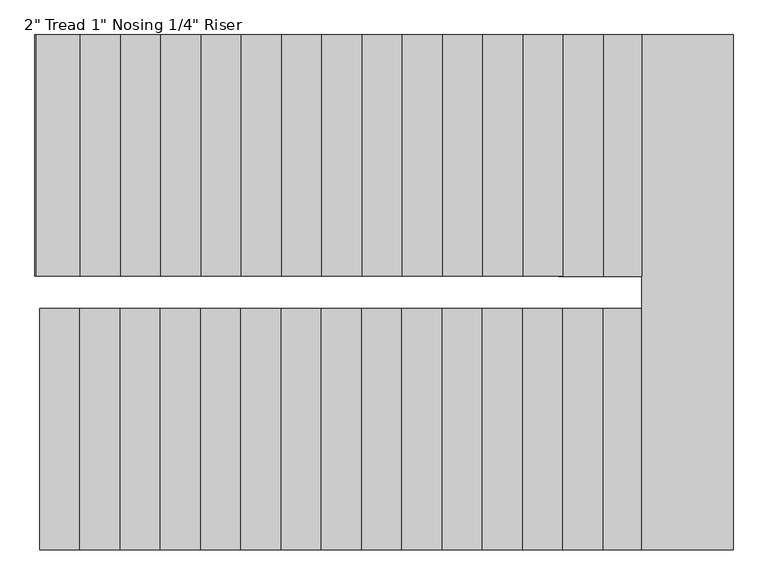
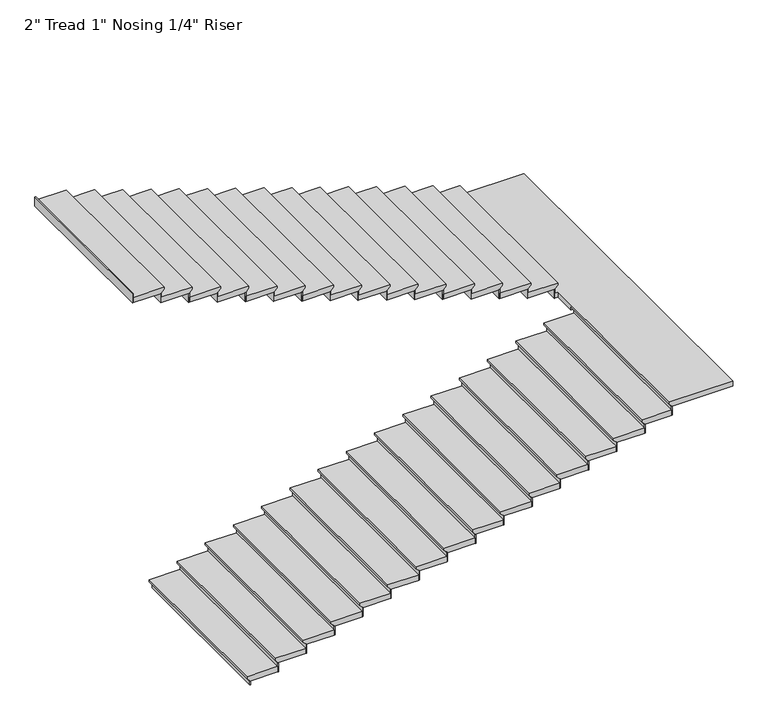
"""IFC4 building model written with IfcOpenShell, lengths in millimetres: stair flight geometry."""

from ifc_helpers import new_model, si_unit, origin, place, context, project, spatial, faceted_brep, source, transform, mapped, element, save


def stair_flight_fd3cf4e0(model_context):
    return source(origin(), model_context, "Body", "Brep", [
        faceted_brep([(1449.3932247, -2065.2659014, 9210.675), (1449.3932247, -2065.2659014, 9229.725), (1449.3932247, -541.2659014, 9229.725), (1449.3932247, -541.2659014, 9210.675), (1474.7932247, -2065.2659014, 9185.275), (1474.7932247, -541.2659014, 9185.275), (1726.3621616, -2065.2659014, 9229.725), (1726.3621616, -541.2659014, 9229.725), (1474.7932247, -541.2659014, 9178.925), (1726.3621616, -541.2659014, 9178.925), (1726.3621616, -2065.2659014, 9178.925), (1474.7932247, -2065.2659014, 9178.925)], [[[0, 1, 2, 3]], [[4, 0, 3, 5]], [[2, 1, 6, 7]], [[8, 9, 10, 11]], [[2, 7, 9, 8, 5, 3]], [[8, 11, 4, 5]], [[6, 1, 0, 4, 11, 10]], [[7, 6, 10, 9]]]),
        faceted_brep([(1474.7932247, -2065.2659014, 9178.925), (1474.7932247, -2065.2659014, 9144.0), (1481.1432247, -2065.2659014, 9144.0), (1481.1432247, -2065.2659014, 9178.925), (1474.7932247, -541.2659014, 9178.925), (1481.1432247, -541.2659014, 9178.925), (1481.1432247, -541.2659014, 9144.0), (1474.7932247, -541.2659014, 9144.0)], [[[0, 1, 2, 3]], [[4, 5, 6, 7]], [[1, 0, 4, 7]], [[2, 1, 7, 6]], [[3, 2, 6, 5]], [[0, 3, 5, 4]]]),
        faceted_brep([(1726.3621616, -2065.2659014, 9264.65), (1726.3621616, -2065.2659014, 9178.925), (1732.7121616, -2065.2659014, 9178.925), (1732.7121616, -2065.2659014, 9264.65), (1726.3621616, -541.2659014, 9264.65), (1732.7121616, -541.2659014, 9264.65), (1732.7121616, -541.2659014, 9178.925), (1726.3621616, -541.2659014, 9178.925)], [[[0, 1, 2, 3]], [[4, 5, 6, 7]], [[1, 0, 4, 7]], [[2, 1, 7, 6]], [[3, 2, 6, 5]], [[0, 3, 5, 4]]]),
        faceted_brep([(1700.9621616, -541.2659014, 9315.45), (1700.9621616, -2065.2659014, 9315.45), (1980.3621616, -2065.2659014, 9315.45), (1980.3621616, -541.2659014, 9315.45), (1726.3621616, -541.2659014, 9264.65), (1980.3621616, -541.2659014, 9264.65), (1980.3621616, -2065.2659014, 9264.65), (1726.3621616, -2065.2659014, 9264.65), (1726.3621616, -541.2659014, 9271.0), (1700.9621616, -541.2659014, 9296.4), (1726.3621616, -2065.2659014, 9271.0), (1700.9621616, -2065.2659014, 9296.4)], [[[0, 1, 2, 3]], [[4, 5, 6, 7]], [[0, 3, 5, 4, 8, 9]], [[4, 7, 10, 8]], [[2, 1, 11, 10, 7, 6]], [[3, 2, 6, 5]], [[11, 1, 0, 9]], [[10, 11, 9, 8]]]),
        faceted_brep([(1980.3621616, -2065.2659014, 9350.375), (1980.3621616, -2065.2659014, 9264.65), (1986.7121616, -2065.2659014, 9264.65), (1986.7121616, -2065.2659014, 9350.375), (1980.3621616, -541.2659014, 9350.375), (1986.7121616, -541.2659014, 9350.375), (1986.7121616, -541.2659014, 9264.65), (1980.3621616, -541.2659014, 9264.65)], [[[0, 1, 2, 3]], [[4, 5, 6, 7]], [[1, 0, 4, 7]], [[2, 1, 7, 6]], [[3, 2, 6, 5]], [[0, 3, 5, 4]]]),
        faceted_brep([(1954.9621616, -541.2659014, 9401.175), (1954.9621616, -2065.2659014, 9401.175), (2234.3621616, -2065.2659014, 9401.175), (2234.3621616, -541.2659014, 9401.175), (1980.3621616, -541.2659014, 9350.375), (2234.3621616, -541.2659014, 9350.375), (2234.3621616, -2065.2659014, 9350.375), (1980.3621616, -2065.2659014, 9350.375), (1980.3621616, -541.2659014, 9356.725), (1954.9621616, -541.2659014, 9382.125), (1980.3621616, -2065.2659014, 9356.725), (1954.9621616, -2065.2659014, 9382.125)], [[[0, 1, 2, 3]], [[4, 5, 6, 7]], [[0, 3, 5, 4, 8, 9]], [[4, 7, 10, 8]], [[2, 1, 11, 10, 7, 6]], [[3, 2, 6, 5]], [[11, 1, 0, 9]], [[10, 11, 9, 8]]]),
        faceted_brep([(2234.3621616, -2065.2659014, 9436.1), (2234.3621616, -2065.2659014, 9350.375), (2240.7121616, -2065.2659014, 9350.375), (2240.7121616, -2065.2659014, 9436.1), (2234.3621616, -541.2659014, 9436.1), (2240.7121616, -541.2659014, 9436.1), (2240.7121616, -541.2659014, 9350.375), (2234.3621616, -541.2659014, 9350.375)], [[[0, 1, 2, 3]], [[4, 5, 6, 7]], [[1, 0, 4, 7]], [[2, 1, 7, 6]], [[3, 2, 6, 5]], [[0, 3, 5, 4]]]),
        faceted_brep([(2208.9621616, -541.2659014, 9486.9), (2208.9621616, -2065.2659014, 9486.9), (2488.3621616, -2065.2659014, 9486.9), (2488.3621616, -541.2659014, 9486.9), (2234.3621616, -541.2659014, 9436.1), (2488.3621616, -541.2659014, 9436.1), (2488.3621616, -2065.2659014, 9436.1), (2234.3621616, -2065.2659014, 9436.1), (2234.3621616, -541.2659014, 9442.45), (2208.9621616, -541.2659014, 9467.85), (2234.3621616, -2065.2659014, 9442.45), (2208.9621616, -2065.2659014, 9467.85)], [[[0, 1, 2, 3]], [[4, 5, 6, 7]], [[0, 3, 5, 4, 8, 9]], [[4, 7, 10, 8]], [[2, 1, 11, 10, 7, 6]], [[3, 2, 6, 5]], [[11, 1, 0, 9]], [[10, 11, 9, 8]]]),
        faceted_brep([(2488.3621616, -2065.2659014, 9521.825), (2488.3621616, -2065.2659014, 9436.1), (2494.7121616, -2065.2659014, 9436.1), (2494.7121616, -2065.2659014, 9521.825), (2488.3621616, -541.2659014, 9521.825), (2494.7121616, -541.2659014, 9521.825), (2494.7121616, -541.2659014, 9436.1), (2488.3621616, -541.2659014, 9436.1)], [[[0, 1, 2, 3]], [[4, 5, 6, 7]], [[1, 0, 4, 7]], [[2, 1, 7, 6]], [[3, 2, 6, 5]], [[0, 3, 5, 4]]]),
        faceted_brep([(2462.9621616, -541.2659014, 9572.625), (2462.9621616, -2065.2659014, 9572.625), (2742.3621616, -2065.2659014, 9572.625), (2742.3621616, -541.2659014, 9572.625), (2488.3621616, -541.2659014, 9521.825), (2742.3621616, -541.2659014, 9521.825), (2742.3621616, -2065.2659014, 9521.825), (2488.3621616, -2065.2659014, 9521.825), (2488.3621616, -541.2659014, 9528.175), (2462.9621616, -541.2659014, 9553.575), (2488.3621616, -2065.2659014, 9528.175), (2462.9621616, -2065.2659014, 9553.575)], [[[0, 1, 2, 3]], [[4, 5, 6, 7]], [[0, 3, 5, 4, 8, 9]], [[4, 7, 10, 8]], [[2, 1, 11, 10, 7, 6]], [[3, 2, 6, 5]], [[11, 1, 0, 9]], [[10, 11, 9, 8]]]),
        faceted_brep([(2742.3621616, -2065.2659014, 9607.55), (2742.3621616, -2065.2659014, 9521.825), (2748.7121616, -2065.2659014, 9521.825), (2748.7121616, -2065.2659014, 9607.55), (2742.3621616, -541.2659014, 9607.55), (2748.7121616, -541.2659014, 9607.55), (2748.7121616, -541.2659014, 9521.825), (2742.3621616, -541.2659014, 9521.825)], [[[0, 1, 2, 3]], [[4, 5, 6, 7]], [[1, 0, 4, 7]], [[2, 1, 7, 6]], [[3, 2, 6, 5]], [[0, 3, 5, 4]]]),
        faceted_brep([(2716.9621616, -541.2659014, 9658.35), (2716.9621616, -2065.2659014, 9658.35), (2996.3621616, -2065.2659014, 9658.35), (2996.3621616, -541.2659014, 9658.35), (2742.3621616, -541.2659014, 9607.55), (2996.3621616, -541.2659014, 9607.55), (2996.3621616, -2065.2659014, 9607.55), (2742.3621616, -2065.2659014, 9607.55), (2742.3621616, -541.2659014, 9613.9), (2716.9621616, -541.2659014, 9639.3), (2742.3621616, -2065.2659014, 9613.9), (2716.9621616, -2065.2659014, 9639.3)], [[[0, 1, 2, 3]], [[4, 5, 6, 7]], [[0, 3, 5, 4, 8, 9]], [[4, 7, 10, 8]], [[2, 1, 11, 10, 7, 6]], [[3, 2, 6, 5]], [[11, 1, 0, 9]], [[10, 11, 9, 8]]]),
        faceted_brep([(2996.3621616, -2065.2659014, 9693.275), (2996.3621616, -2065.2659014, 9607.55), (3002.7121616, -2065.2659014, 9607.55), (3002.7121616, -2065.2659014, 9693.275), (2996.3621616, -541.2659014, 9693.275), (3002.7121616, -541.2659014, 9693.275), (3002.7121616, -541.2659014, 9607.55), (2996.3621616, -541.2659014, 9607.55)], [[[0, 1, 2, 3]], [[4, 5, 6, 7]], [[1, 0, 4, 7]], [[2, 1, 7, 6]], [[3, 2, 6, 5]], [[0, 3, 5, 4]]]),
        faceted_brep([(2970.9621616, -541.2659014, 9744.075), (2970.9621616, -2065.2659014, 9744.075), (3250.3621616, -2065.2659014, 9744.075), (3250.3621616, -541.2659014, 9744.075), (2996.3621616, -541.2659014, 9693.275), (3250.3621616, -541.2659014, 9693.275), (3250.3621616, -2065.2659014, 9693.275), (2996.3621616, -2065.2659014, 9693.275), (2996.3621616, -541.2659014, 9699.625), (2970.9621616, -541.2659014, 9725.025), (2996.3621616, -2065.2659014, 9699.625), (2970.9621616, -2065.2659014, 9725.025)], [[[0, 1, 2, 3]], [[4, 5, 6, 7]], [[0, 3, 5, 4, 8, 9]], [[4, 7, 10, 8]], [[2, 1, 11, 10, 7, 6]], [[3, 2, 6, 5]], [[11, 1, 0, 9]], [[10, 11, 9, 8]]]),
        faceted_brep([(3250.3621616, -2065.2659014, 9779.0), (3250.3621616, -2065.2659014, 9693.275), (3256.7121616, -2065.2659014, 9693.275), (3256.7121616, -2065.2659014, 9779.0), (3250.3621616, -541.2659014, 9779.0), (3256.7121616, -541.2659014, 9779.0), (3256.7121616, -541.2659014, 9693.275), (3250.3621616, -541.2659014, 9693.275)], [[[0, 1, 2, 3]], [[4, 5, 6, 7]], [[1, 0, 4, 7]], [[2, 1, 7, 6]], [[3, 2, 6, 5]], [[0, 3, 5, 4]]]),
        faceted_brep([(3224.9621616, -541.2659014, 9829.8), (3224.9621616, -2065.2659014, 9829.8), (3504.3621616, -2065.2659014, 9829.8), (3504.3621616, -541.2659014, 9829.8), (3250.3621616, -541.2659014, 9779.0), (3504.3621616, -541.2659014, 9779.0), (3504.3621616, -2065.2659014, 9779.0), (3250.3621616, -2065.2659014, 9779.0), (3250.3621616, -541.2659014, 9785.35), (3224.9621616, -541.2659014, 9810.75), (3250.3621616, -2065.2659014, 9785.35), (3224.9621616, -2065.2659014, 9810.75)], [[[0, 1, 2, 3]], [[4, 5, 6, 7]], [[0, 3, 5, 4, 8, 9]], [[4, 7, 10, 8]], [[2, 1, 11, 10, 7, 6]], [[3, 2, 6, 5]], [[11, 1, 0, 9]], [[10, 11, 9, 8]]]),
        faceted_brep([(3504.3621616, -2065.2659014, 9864.725), (3504.3621616, -2065.2659014, 9779.0), (3510.7121616, -2065.2659014, 9779.0), (3510.7121616, -2065.2659014, 9864.725), (3504.3621616, -541.2659014, 9864.725), (3510.7121616, -541.2659014, 9864.725), (3510.7121616, -541.2659014, 9779.0), (3504.3621616, -541.2659014, 9779.0)], [[[0, 1, 2, 3]], [[4, 5, 6, 7]], [[1, 0, 4, 7]], [[2, 1, 7, 6]], [[3, 2, 6, 5]], [[0, 3, 5, 4]]]),
        faceted_brep([(3478.9621616, -541.2659014, 9915.525), (3478.9621616, -2065.2659014, 9915.525), (3758.3621616, -2065.2659014, 9915.525), (3758.3621616, -541.2659014, 9915.525), (3504.3621616, -541.2659014, 9864.725), (3758.3621616, -541.2659014, 9864.725), (3758.3621616, -2065.2659014, 9864.725), (3504.3621616, -2065.2659014, 9864.725), (3504.3621616, -541.2659014, 9871.075), (3478.9621616, -541.2659014, 9896.475), (3504.3621616, -2065.2659014, 9871.075), (3478.9621616, -2065.2659014, 9896.475)], [[[0, 1, 2, 3]], [[4, 5, 6, 7]], [[0, 3, 5, 4, 8, 9]], [[4, 7, 10, 8]], [[2, 1, 11, 10, 7, 6]], [[3, 2, 6, 5]], [[11, 1, 0, 9]], [[10, 11, 9, 8]]]),
        faceted_brep([(3758.3621616, -2065.2659014, 9950.45), (3758.3621616, -2065.2659014, 9864.725), (3764.7121616, -2065.2659014, 9864.725), (3764.7121616, -2065.2659014, 9950.45), (3758.3621616, -541.2659014, 9950.45), (3764.7121616, -541.2659014, 9950.45), (3764.7121616, -541.2659014, 9864.725), (3758.3621616, -541.2659014, 9864.725)], [[[0, 1, 2, 3]], [[4, 5, 6, 7]], [[1, 0, 4, 7]], [[2, 1, 7, 6]], [[3, 2, 6, 5]], [[0, 3, 5, 4]]]),
        faceted_brep([(3732.9621616, -541.2659014, 10001.25), (3732.9621616, -2065.2659014, 10001.25), (4012.3621616, -2065.2659014, 10001.25), (4012.3621616, -541.2659014, 10001.25), (3758.3621616, -541.2659014, 9950.45), (4012.3621616, -541.2659014, 9950.45), (4012.3621616, -2065.2659014, 9950.45), (3758.3621616, -2065.2659014, 9950.45), (3758.3621616, -541.2659014, 9956.8), (3732.9621616, -541.2659014, 9982.2), (3758.3621616, -2065.2659014, 9956.8), (3732.9621616, -2065.2659014, 9982.2)], [[[0, 1, 2, 3]], [[4, 5, 6, 7]], [[0, 3, 5, 4, 8, 9]], [[4, 7, 10, 8]], [[2, 1, 11, 10, 7, 6]], [[3, 2, 6, 5]], [[11, 1, 0, 9]], [[10, 11, 9, 8]]]),
        faceted_brep([(4012.3621616, -2065.2659014, 10036.175), (4012.3621616, -2065.2659014, 9950.45), (4018.7121616, -2065.2659014, 9950.45), (4018.7121616, -2065.2659014, 10036.175), (4012.3621616, -541.2659014, 10036.175), (4018.7121616, -541.2659014, 10036.175), (4018.7121616, -541.2659014, 9950.45), (4012.3621616, -541.2659014, 9950.45)], [[[0, 1, 2, 3]], [[4, 5, 6, 7]], [[1, 0, 4, 7]], [[2, 1, 7, 6]], [[3, 2, 6, 5]], [[0, 3, 5, 4]]]),
        faceted_brep([(3986.9621616, -541.2659014, 10086.975), (3986.9621616, -2065.2659014, 10086.975), (4266.3621616, -2065.2659014, 10086.975), (4266.3621616, -541.2659014, 10086.975), (4012.3621616, -541.2659014, 10036.175), (4266.3621616, -541.2659014, 10036.175), (4266.3621616, -2065.2659014, 10036.175), (4012.3621616, -2065.2659014, 10036.175), (4012.3621616, -541.2659014, 10042.525), (3986.9621616, -541.2659014, 10067.925), (4012.3621616, -2065.2659014, 10042.525), (3986.9621616, -2065.2659014, 10067.925)], [[[0, 1, 2, 3]], [[4, 5, 6, 7]], [[0, 3, 5, 4, 8, 9]], [[4, 7, 10, 8]], [[2, 1, 11, 10, 7, 6]], [[3, 2, 6, 5]], [[11, 1, 0, 9]], [[10, 11, 9, 8]]]),
        faceted_brep([(4266.3621616, -2065.2659014, 10121.9), (4266.3621616, -2065.2659014, 10036.175), (4272.7121616, -2065.2659014, 10036.175), (4272.7121616, -2065.2659014, 10121.9), (4266.3621616, -541.2659014, 10121.9), (4272.7121616, -541.2659014, 10121.9), (4272.7121616, -541.2659014, 10036.175), (4266.3621616, -541.2659014, 10036.175)], [[[0, 1, 2, 3]], [[4, 5, 6, 7]], [[1, 0, 4, 7]], [[2, 1, 7, 6]], [[3, 2, 6, 5]], [[0, 3, 5, 4]]]),
        faceted_brep([(4240.9621616, -541.2659014, 10172.7), (4240.9621616, -2065.2659014, 10172.7), (4520.3621616, -2065.2659014, 10172.7), (4520.3621616, -541.2659014, 10172.7), (4266.3621616, -541.2659014, 10121.9), (4520.3621616, -541.2659014, 10121.9), (4520.3621616, -2065.2659014, 10121.9), (4266.3621616, -2065.2659014, 10121.9), (4266.3621616, -541.2659014, 10128.25), (4240.9621616, -541.2659014, 10153.65), (4266.3621616, -2065.2659014, 10128.25), (4240.9621616, -2065.2659014, 10153.65)], [[[0, 1, 2, 3]], [[4, 5, 6, 7]], [[0, 3, 5, 4, 8, 9]], [[4, 7, 10, 8]], [[2, 1, 11, 10, 7, 6]], [[3, 2, 6, 5]], [[11, 1, 0, 9]], [[10, 11, 9, 8]]]),
        faceted_brep([(4520.3621616, -2065.2659014, 10207.625), (4520.3621616, -2065.2659014, 10121.9), (4526.7121616, -2065.2659014, 10121.9), (4526.7121616, -2065.2659014, 10207.625), (4520.3621616, -541.2659014, 10207.625), (4526.7121616, -541.2659014, 10207.625), (4526.7121616, -541.2659014, 10121.9), (4520.3621616, -541.2659014, 10121.9)], [[[0, 1, 2, 3]], [[4, 5, 6, 7]], [[1, 0, 4, 7]], [[2, 1, 7, 6]], [[3, 2, 6, 5]], [[0, 3, 5, 4]]]),
        faceted_brep([(4494.9621616, -541.2659014, 10258.425), (4494.9621616, -2065.2659014, 10258.425), (4774.3621616, -2065.2659014, 10258.425), (4774.3621616, -541.2659014, 10258.425), (4520.3621616, -541.2659014, 10207.625), (4774.3621616, -541.2659014, 10207.625), (4774.3621616, -2065.2659014, 10207.625), (4520.3621616, -2065.2659014, 10207.625), (4520.3621616, -541.2659014, 10213.975), (4494.9621616, -541.2659014, 10239.375), (4520.3621616, -2065.2659014, 10213.975), (4494.9621616, -2065.2659014, 10239.375)], [[[0, 1, 2, 3]], [[4, 5, 6, 7]], [[0, 3, 5, 4, 8, 9]], [[4, 7, 10, 8]], [[2, 1, 11, 10, 7, 6]], [[3, 2, 6, 5]], [[11, 1, 0, 9]], [[10, 11, 9, 8]]]),
        faceted_brep([(4774.3621616, -2065.2659014, 10293.35), (4774.3621616, -2065.2659014, 10207.625), (4780.7121616, -2065.2659014, 10207.625), (4780.7121616, -2065.2659014, 10293.35), (4774.3621616, -541.2659014, 10293.35), (4780.7121616, -541.2659014, 10293.35), (4780.7121616, -541.2659014, 10207.625), (4774.3621616, -541.2659014, 10207.625)], [[[0, 1, 2, 3]], [[4, 5, 6, 7]], [[1, 0, 4, 7]], [[2, 1, 7, 6]], [[3, 2, 6, 5]], [[0, 3, 5, 4]]]),
        faceted_brep([(4748.9621616, -541.2659014, 10344.15), (4748.9621616, -2065.2659014, 10344.15), (5028.3621616, -2065.2659014, 10344.15), (5028.3621616, -541.2659014, 10344.15), (4774.3621616, -541.2659014, 10293.35), (5028.3621616, -541.2659014, 10293.35), (5028.3621616, -2065.2659014, 10293.35), (4774.3621616, -2065.2659014, 10293.35), (4774.3621616, -541.2659014, 10299.7), (4748.9621616, -541.2659014, 10325.1), (4774.3621616, -2065.2659014, 10299.7), (4748.9621616, -2065.2659014, 10325.1)], [[[0, 1, 2, 3]], [[4, 5, 6, 7]], [[0, 3, 5, 4, 8, 9]], [[4, 7, 10, 8]], [[2, 1, 11, 10, 7, 6]], [[3, 2, 6, 5]], [[11, 1, 0, 9]], [[10, 11, 9, 8]]]),
        faceted_brep([(5028.3621616, -2065.2659014, 10379.075), (5028.3621616, -2065.2659014, 10293.35), (5034.7121616, -2065.2659014, 10293.35), (5034.7121616, -2065.2659014, 10379.075), (5028.3621616, -541.2659014, 10379.075), (5034.7121616, -541.2659014, 10379.075), (5034.7121616, -541.2659014, 10293.35), (5028.3621616, -541.2659014, 10293.35)], [[[0, 1, 2, 3]], [[4, 5, 6, 7]], [[1, 0, 4, 7]], [[2, 1, 7, 6]], [[3, 2, 6, 5]], [[0, 3, 5, 4]]]),
        faceted_brep([(5002.9621616, -541.2659014, 10429.875), (5002.9621616, -2065.2659014, 10429.875), (5272.0669505, -2065.2659014, 10429.875), (5272.0669505, -541.2659014, 10429.875), (5028.3621616, -541.2659014, 10379.075), (5272.0669505, -541.2659014, 10379.075), (5272.0669505, -2065.2659014, 10379.075), (5028.3621616, -2065.2659014, 10379.075), (5028.3621616, -541.2659014, 10385.425), (5002.9621616, -541.2659014, 10410.825), (5028.3621616, -2065.2659014, 10385.425), (5002.9621616, -2065.2659014, 10410.825)], [[[0, 1, 2, 3]], [[4, 5, 6, 7]], [[0, 3, 5, 4, 8, 9]], [[4, 7, 10, 8]], [[2, 1, 11, 10, 7, 6]], [[3, 2, 6, 5]], [[11, 1, 0, 9]], [[10, 11, 9, 8]]]),
        faceted_brep([(5272.0669505, -2065.2659014, 10464.8), (5272.0669505, -2065.2659014, 10379.075), (5278.4169505, -2065.2659014, 10379.075), (5278.4169505, -2065.2659014, 10464.8), (5272.0669505, -541.2659014, 10464.8), (5278.4169505, -541.2659014, 10464.8), (5278.4169505, -541.2659014, 10379.075), (5272.0669505, -541.2659014, 10379.075)], [[[0, 1, 2, 3]], [[4, 5, 6, 7]], [[1, 0, 4, 7]], [[2, 1, 7, 6]], [[3, 2, 6, 5]], [[0, 3, 5, 4]]]),
        faceted_brep([(5221.2669505, -337.9910016, 10515.6), (5246.6669505, -337.9910016, 10515.6), (5246.6669505, -2065.2659014, 10515.6), (5822.2548051, -2065.2659014, 10515.6), (5822.2548051, 1185.9340986, 10515.6), (5221.2669505, 1185.9340986, 10515.6), (5246.6669505, -337.9910016, 10464.8), (5221.2669505, -337.9910016, 10464.8), (5221.2669505, 1185.9340986, 10464.8), (5822.2548051, 1185.9340986, 10464.8), (5822.2548051, -2065.2659014, 10464.8), (5272.0669505, -2065.2659014, 10464.8), (5272.0669505, -541.2659014, 10464.8), (5246.6669505, -541.2659014, 10464.8), (5246.6669505, -541.2659014, 10496.55), (5246.6669505, -2065.2659014, 10496.55), (5272.0669505, -541.2659014, 10471.15), (5272.0669505, -2065.2659014, 10471.15)], [[[0, 1, 2, 3, 4, 5]], [[6, 7, 8, 9, 10, 11, 12, 13]], [[1, 0, 7, 6]], [[2, 1, 6, 13, 14, 15]], [[13, 12, 16, 14]], [[12, 11, 17, 16]], [[3, 2, 15, 17, 11, 10]], [[4, 3, 10, 9]], [[5, 4, 9, 8]], [[0, 5, 8, 7]], [[17, 15, 14, 16]]]),
        faceted_brep([(5221.2669505, 1185.9340986, 10550.525), (5221.2669505, 1185.9340986, 10464.8), (5214.9169505, 1185.9340986, 10464.8), (5214.9169505, 1185.9340986, 10550.525), (5221.2669505, -337.9910016, 10550.525), (5214.9169505, -337.9910016, 10550.525), (5214.9169505, -337.9910016, 10464.8), (5221.2669505, -337.9910016, 10464.8)], [[[0, 1, 2, 3]], [[4, 5, 6, 7]], [[1, 0, 4, 7]], [[2, 1, 7, 6]], [[3, 2, 6, 5]], [[0, 3, 5, 4]]]),
        faceted_brep([(5246.6669505, -337.9910016, 10601.325), (5246.6669505, 1185.9340986, 10601.325), (4977.5621616, 1185.9340986, 10601.325), (4977.5621616, -337.9910016, 10601.325), (5221.2669505, -337.9910016, 10550.525), (4977.5621616, -337.9910016, 10550.525), (4977.5621616, 1185.9340986, 10550.525), (5221.2669505, 1185.9340986, 10550.525), (5221.2669505, -337.9910016, 10556.875), (5246.6669505, -337.9910016, 10582.275), (5221.2669505, 1185.9340986, 10556.875), (5246.6669505, 1185.9340986, 10582.275)], [[[0, 1, 2, 3]], [[4, 5, 6, 7]], [[0, 3, 5, 4, 8, 9]], [[4, 7, 10, 8]], [[2, 1, 11, 10, 7, 6]], [[3, 2, 6, 5]], [[11, 1, 0, 9]], [[10, 11, 9, 8]]]),
        faceted_brep([(4977.5621616, 1185.9340986, 10636.25), (4977.5621616, 1185.9340986, 10550.525), (4971.2121616, 1185.9340986, 10550.525), (4971.2121616, 1185.9340986, 10636.25), (4977.5621616, -337.9910016, 10636.25), (4971.2121616, -337.9910016, 10636.25), (4971.2121616, -337.9910016, 10550.525), (4977.5621616, -337.9910016, 10550.525)], [[[0, 1, 2, 3]], [[4, 5, 6, 7]], [[1, 0, 4, 7]], [[2, 1, 7, 6]], [[3, 2, 6, 5]], [[0, 3, 5, 4]]]),
        faceted_brep([(5002.9621616, -337.9910016, 10687.05), (5002.9621616, 1185.9340986, 10687.05), (4723.5621616, 1185.9340986, 10687.05), (4723.5621616, -337.9910016, 10687.05), (4977.5621616, -337.9910016, 10636.25), (4723.5621616, -337.9910016, 10636.25), (4723.5621616, 1185.9340986, 10636.25), (4977.5621616, 1185.9340986, 10636.25), (4977.5621616, -337.9910016, 10642.6), (5002.9621616, -337.9910016, 10668.0), (4977.5621616, 1185.9340986, 10642.6), (5002.9621616, 1185.9340986, 10668.0)], [[[0, 1, 2, 3]], [[4, 5, 6, 7]], [[0, 3, 5, 4, 8, 9]], [[4, 7, 10, 8]], [[2, 1, 11, 10, 7, 6]], [[3, 2, 6, 5]], [[11, 1, 0, 9]], [[10, 11, 9, 8]]]),
        faceted_brep([(4723.5621616, 1185.9340986, 10721.975), (4723.5621616, 1185.9340986, 10636.25), (4717.2121616, 1185.9340986, 10636.25), (4717.2121616, 1185.9340986, 10721.975), (4723.5621616, -337.9910016, 10721.975), (4717.2121616, -337.9910016, 10721.975), (4717.2121616, -337.9910016, 10636.25), (4723.5621616, -337.9910016, 10636.25)], [[[0, 1, 2, 3]], [[4, 5, 6, 7]], [[1, 0, 4, 7]], [[2, 1, 7, 6]], [[3, 2, 6, 5]], [[0, 3, 5, 4]]]),
        faceted_brep([(4748.9621616, -337.9910016, 10772.775), (4748.9621616, 1185.9340986, 10772.775), (4469.5621616, 1185.9340986, 10772.775), (4469.5621616, -337.9910016, 10772.775), (4723.5621616, -337.9910016, 10721.975), (4469.5621616, -337.9910016, 10721.975), (4469.5621616, 1185.9340986, 10721.975), (4723.5621616, 1185.9340986, 10721.975), (4723.5621616, -337.9910016, 10728.325), (4748.9621616, -337.9910016, 10753.725), (4723.5621616, 1185.9340986, 10728.325), (4748.9621616, 1185.9340986, 10753.725)], [[[0, 1, 2, 3]], [[4, 5, 6, 7]], [[0, 3, 5, 4, 8, 9]], [[4, 7, 10, 8]], [[2, 1, 11, 10, 7, 6]], [[3, 2, 6, 5]], [[11, 1, 0, 9]], [[10, 11, 9, 8]]]),
        faceted_brep([(4469.5621616, 1185.9340986, 10807.7), (4469.5621616, 1185.9340986, 10721.975), (4463.2121616, 1185.9340986, 10721.975), (4463.2121616, 1185.9340986, 10807.7), (4469.5621616, -337.9910016, 10807.7), (4463.2121616, -337.9910016, 10807.7), (4463.2121616, -337.9910016, 10721.975), (4469.5621616, -337.9910016, 10721.975)], [[[0, 1, 2, 3]], [[4, 5, 6, 7]], [[1, 0, 4, 7]], [[2, 1, 7, 6]], [[3, 2, 6, 5]], [[0, 3, 5, 4]]]),
        faceted_brep([(4494.9621616, -337.9910016, 10858.5), (4494.9621616, 1185.9340986, 10858.5), (4215.5621616, 1185.9340986, 10858.5), (4215.5621616, -337.9910016, 10858.5), (4469.5621616, -337.9910016, 10807.7), (4215.5621616, -337.9910016, 10807.7), (4215.5621616, 1185.9340986, 10807.7), (4469.5621616, 1185.9340986, 10807.7), (4469.5621616, -337.9910016, 10814.05), (4494.9621616, -337.9910016, 10839.45), (4469.5621616, 1185.9340986, 10814.05), (4494.9621616, 1185.9340986, 10839.45)], [[[0, 1, 2, 3]], [[4, 5, 6, 7]], [[0, 3, 5, 4, 8, 9]], [[4, 7, 10, 8]], [[2, 1, 11, 10, 7, 6]], [[3, 2, 6, 5]], [[11, 1, 0, 9]], [[10, 11, 9, 8]]]),
        faceted_brep([(4215.5621616, 1185.9340986, 10893.425), (4215.5621616, 1185.9340986, 10807.7), (4209.2121616, 1185.9340986, 10807.7), (4209.2121616, 1185.9340986, 10893.425), (4215.5621616, -337.9910016, 10893.425), (4209.2121616, -337.9910016, 10893.425), (4209.2121616, -337.9910016, 10807.7), (4215.5621616, -337.9910016, 10807.7)], [[[0, 1, 2, 3]], [[4, 5, 6, 7]], [[1, 0, 4, 7]], [[2, 1, 7, 6]], [[3, 2, 6, 5]], [[0, 3, 5, 4]]]),
        faceted_brep([(4240.9621616, -337.9910016, 10944.225), (4240.9621616, 1185.9340986, 10944.225), (3961.5621616, 1185.9340986, 10944.225), (3961.5621616, -337.9910016, 10944.225), (4215.5621616, -337.9910016, 10893.425), (3961.5621616, -337.9910016, 10893.425), (3961.5621616, 1185.9340986, 10893.425), (4215.5621616, 1185.9340986, 10893.425), (4215.5621616, -337.9910016, 10899.775), (4240.9621616, -337.9910016, 10925.175), (4215.5621616, 1185.9340986, 10899.775), (4240.9621616, 1185.9340986, 10925.175)], [[[0, 1, 2, 3]], [[4, 5, 6, 7]], [[0, 3, 5, 4, 8, 9]], [[4, 7, 10, 8]], [[2, 1, 11, 10, 7, 6]], [[3, 2, 6, 5]], [[11, 1, 0, 9]], [[10, 11, 9, 8]]]),
        faceted_brep([(3961.5621616, 1185.9340986, 10979.15), (3961.5621616, 1185.9340986, 10893.425), (3955.2121616, 1185.9340986, 10893.425), (3955.2121616, 1185.9340986, 10979.15), (3961.5621616, -337.9910016, 10979.15), (3955.2121616, -337.9910016, 10979.15), (3955.2121616, -337.9910016, 10893.425), (3961.5621616, -337.9910016, 10893.425)], [[[0, 1, 2, 3]], [[4, 5, 6, 7]], [[1, 0, 4, 7]], [[2, 1, 7, 6]], [[3, 2, 6, 5]], [[0, 3, 5, 4]]]),
        faceted_brep([(3986.9621616, -337.9910016, 11029.95), (3986.9621616, 1185.9340986, 11029.95), (3707.5621616, 1185.9340986, 11029.95), (3707.5621616, -337.9910016, 11029.95), (3961.5621616, -337.9910016, 10979.15), (3707.5621616, -337.9910016, 10979.15), (3707.5621616, 1185.9340986, 10979.15), (3961.5621616, 1185.9340986, 10979.15), (3961.5621616, -337.9910016, 10985.5), (3986.9621616, -337.9910016, 11010.9), (3961.5621616, 1185.9340986, 10985.5), (3986.9621616, 1185.9340986, 11010.9)], [[[0, 1, 2, 3]], [[4, 5, 6, 7]], [[0, 3, 5, 4, 8, 9]], [[4, 7, 10, 8]], [[2, 1, 11, 10, 7, 6]], [[3, 2, 6, 5]], [[11, 1, 0, 9]], [[10, 11, 9, 8]]]),
        faceted_brep([(3707.5621616, 1185.9340986, 11064.875), (3707.5621616, 1185.9340986, 10979.15), (3701.2121616, 1185.9340986, 10979.15), (3701.2121616, 1185.9340986, 11064.875), (3707.5621616, -337.9910016, 11064.875), (3701.2121616, -337.9910016, 11064.875), (3701.2121616, -337.9910016, 10979.15), (3707.5621616, -337.9910016, 10979.15)], [[[0, 1, 2, 3]], [[4, 5, 6, 7]], [[1, 0, 4, 7]], [[2, 1, 7, 6]], [[3, 2, 6, 5]], [[0, 3, 5, 4]]]),
        faceted_brep([(3732.9621616, -337.9910016, 11115.675), (3732.9621616, 1185.9340986, 11115.675), (3453.5621616, 1185.9340986, 11115.675), (3453.5621616, -337.9910016, 11115.675), (3707.5621616, -337.9910016, 11064.875), (3453.5621616, -337.9910016, 11064.875), (3453.5621616, 1185.9340986, 11064.875), (3707.5621616, 1185.9340986, 11064.875), (3707.5621616, -337.9910016, 11071.225), (3732.9621616, -337.9910016, 11096.625), (3707.5621616, 1185.9340986, 11071.225), (3732.9621616, 1185.9340986, 11096.625)], [[[0, 1, 2, 3]], [[4, 5, 6, 7]], [[0, 3, 5, 4, 8, 9]], [[4, 7, 10, 8]], [[2, 1, 11, 10, 7, 6]], [[3, 2, 6, 5]], [[11, 1, 0, 9]], [[10, 11, 9, 8]]]),
        faceted_brep([(3453.5621616, 1185.9340986, 11150.6), (3453.5621616, 1185.9340986, 11064.875), (3447.2121616, 1185.9340986, 11064.875), (3447.2121616, 1185.9340986, 11150.6), (3453.5621616, -337.9910016, 11150.6), (3447.2121616, -337.9910016, 11150.6), (3447.2121616, -337.9910016, 11064.875), (3453.5621616, -337.9910016, 11064.875)], [[[0, 1, 2, 3]], [[4, 5, 6, 7]], [[1, 0, 4, 7]], [[2, 1, 7, 6]], [[3, 2, 6, 5]], [[0, 3, 5, 4]]]),
        faceted_brep([(3478.9621616, -337.9910016, 11201.4), (3478.9621616, 1185.9340986, 11201.4), (3199.5621616, 1185.9340986, 11201.4), (3199.5621616, -337.9910016, 11201.4), (3453.5621616, -337.9910016, 11150.6), (3199.5621616, -337.9910016, 11150.6), (3199.5621616, 1185.9340986, 11150.6), (3453.5621616, 1185.9340986, 11150.6), (3453.5621616, -337.9910016, 11156.95), (3478.9621616, -337.9910016, 11182.35), (3453.5621616, 1185.9340986, 11156.95), (3478.9621616, 1185.9340986, 11182.35)], [[[0, 1, 2, 3]], [[4, 5, 6, 7]], [[0, 3, 5, 4, 8, 9]], [[4, 7, 10, 8]], [[2, 1, 11, 10, 7, 6]], [[3, 2, 6, 5]], [[11, 1, 0, 9]], [[10, 11, 9, 8]]]),
        faceted_brep([(3199.5621616, 1185.9340986, 11236.325), (3199.5621616, 1185.9340986, 11150.6), (3193.2121616, 1185.9340986, 11150.6), (3193.2121616, 1185.9340986, 11236.325), (3199.5621616, -337.9910016, 11236.325), (3193.2121616, -337.9910016, 11236.325), (3193.2121616, -337.9910016, 11150.6), (3199.5621616, -337.9910016, 11150.6)], [[[0, 1, 2, 3]], [[4, 5, 6, 7]], [[1, 0, 4, 7]], [[2, 1, 7, 6]], [[3, 2, 6, 5]], [[0, 3, 5, 4]]]),
        faceted_brep([(3224.9621616, -337.9910016, 11287.125), (3224.9621616, 1185.9340986, 11287.125), (2945.5621616, 1185.9340986, 11287.125), (2945.5621616, -337.9910016, 11287.125), (3199.5621616, -337.9910016, 11236.325), (2945.5621616, -337.9910016, 11236.325), (2945.5621616, 1185.9340986, 11236.325), (3199.5621616, 1185.9340986, 11236.325), (3199.5621616, -337.9910016, 11242.675), (3224.9621616, -337.9910016, 11268.075), (3199.5621616, 1185.9340986, 11242.675), (3224.9621616, 1185.9340986, 11268.075)], [[[0, 1, 2, 3]], [[4, 5, 6, 7]], [[0, 3, 5, 4, 8, 9]], [[4, 7, 10, 8]], [[2, 1, 11, 10, 7, 6]], [[3, 2, 6, 5]], [[11, 1, 0, 9]], [[10, 11, 9, 8]]]),
        faceted_brep([(2945.5621616, 1185.9340986, 11322.05), (2945.5621616, 1185.9340986, 11236.325), (2939.2121616, 1185.9340986, 11236.325), (2939.2121616, 1185.9340986, 11322.05), (2945.5621616, -337.9910016, 11322.05), (2939.2121616, -337.9910016, 11322.05), (2939.2121616, -337.9910016, 11236.325), (2945.5621616, -337.9910016, 11236.325)], [[[0, 1, 2, 3]], [[4, 5, 6, 7]], [[1, 0, 4, 7]], [[2, 1, 7, 6]], [[3, 2, 6, 5]], [[0, 3, 5, 4]]]),
        faceted_brep([(2970.9621616, -337.9910016, 11372.85), (2970.9621616, 1185.9340986, 11372.85), (2691.5621616, 1185.9340986, 11372.85), (2691.5621616, -337.9910016, 11372.85), (2945.5621616, -337.9910016, 11322.05), (2691.5621616, -337.9910016, 11322.05), (2691.5621616, 1185.9340986, 11322.05), (2945.5621616, 1185.9340986, 11322.05), (2945.5621616, -337.9910016, 11328.4), (2970.9621616, -337.9910016, 11353.8), (2945.5621616, 1185.9340986, 11328.4), (2970.9621616, 1185.9340986, 11353.8)], [[[0, 1, 2, 3]], [[4, 5, 6, 7]], [[0, 3, 5, 4, 8, 9]], [[4, 7, 10, 8]], [[2, 1, 11, 10, 7, 6]], [[3, 2, 6, 5]], [[11, 1, 0, 9]], [[10, 11, 9, 8]]]),
        faceted_brep([(2691.5621616, 1185.9340986, 11407.775), (2691.5621616, 1185.9340986, 11322.05), (2685.2121616, 1185.9340986, 11322.05), (2685.2121616, 1185.9340986, 11407.775), (2691.5621616, -337.9910016, 11407.775), (2685.2121616, -337.9910016, 11407.775), (2685.2121616, -337.9910016, 11322.05), (2691.5621616, -337.9910016, 11322.05)], [[[0, 1, 2, 3]], [[4, 5, 6, 7]], [[1, 0, 4, 7]], [[2, 1, 7, 6]], [[3, 2, 6, 5]], [[0, 3, 5, 4]]]),
        faceted_brep([(2716.9621616, -337.9910016, 11458.575), (2716.9621616, 1185.9340986, 11458.575), (2437.5621616, 1185.9340986, 11458.575), (2437.5621616, -337.9910016, 11458.575), (2691.5621616, -337.9910016, 11407.775), (2437.5621616, -337.9910016, 11407.775), (2437.5621616, 1185.9340986, 11407.775), (2691.5621616, 1185.9340986, 11407.775), (2691.5621616, -337.9910016, 11414.125), (2716.9621616, -337.9910016, 11439.525), (2691.5621616, 1185.9340986, 11414.125), (2716.9621616, 1185.9340986, 11439.525)], [[[0, 1, 2, 3]], [[4, 5, 6, 7]], [[0, 3, 5, 4, 8, 9]], [[4, 7, 10, 8]], [[2, 1, 11, 10, 7, 6]], [[3, 2, 6, 5]], [[11, 1, 0, 9]], [[10, 11, 9, 8]]]),
        faceted_brep([(2437.5621616, 1185.9340986, 11493.5), (2437.5621616, 1185.9340986, 11407.775), (2431.2121616, 1185.9340986, 11407.775), (2431.2121616, 1185.9340986, 11493.5), (2437.5621616, -337.9910016, 11493.5), (2431.2121616, -337.9910016, 11493.5), (2431.2121616, -337.9910016, 11407.775), (2437.5621616, -337.9910016, 11407.775)], [[[0, 1, 2, 3]], [[4, 5, 6, 7]], [[1, 0, 4, 7]], [[2, 1, 7, 6]], [[3, 2, 6, 5]], [[0, 3, 5, 4]]]),
        faceted_brep([(2462.9621616, -337.9910016, 11544.3), (2462.9621616, 1185.9340986, 11544.3), (2183.5621616, 1185.9340986, 11544.3), (2183.5621616, -337.9910016, 11544.3), (2437.5621616, -337.9910016, 11493.5), (2183.5621616, -337.9910016, 11493.5), (2183.5621616, 1185.9340986, 11493.5), (2437.5621616, 1185.9340986, 11493.5), (2437.5621616, -337.9910016, 11499.85), (2462.9621616, -337.9910016, 11525.25), (2437.5621616, 1185.9340986, 11499.85), (2462.9621616, 1185.9340986, 11525.25)], [[[0, 1, 2, 3]], [[4, 5, 6, 7]], [[0, 3, 5, 4, 8, 9]], [[4, 7, 10, 8]], [[2, 1, 11, 10, 7, 6]], [[3, 2, 6, 5]], [[11, 1, 0, 9]], [[10, 11, 9, 8]]]),
        faceted_brep([(2183.5621616, 1185.9340986, 11579.225), (2183.5621616, 1185.9340986, 11493.5), (2177.2121616, 1185.9340986, 11493.5), (2177.2121616, 1185.9340986, 11579.225), (2183.5621616, -337.9910016, 11579.225), (2177.2121616, -337.9910016, 11579.225), (2177.2121616, -337.9910016, 11493.5), (2183.5621616, -337.9910016, 11493.5)], [[[0, 1, 2, 3]], [[4, 5, 6, 7]], [[1, 0, 4, 7]], [[2, 1, 7, 6]], [[3, 2, 6, 5]], [[0, 3, 5, 4]]]),
        faceted_brep([(2208.9621616, -337.9910016, 11630.025), (2208.9621616, 1185.9340986, 11630.025), (1929.5621616, 1185.9340986, 11630.025), (1929.5621616, -337.9910016, 11630.025), (2183.5621616, -337.9910016, 11579.225), (1929.5621616, -337.9910016, 11579.225), (1929.5621616, 1185.9340986, 11579.225), (2183.5621616, 1185.9340986, 11579.225), (2183.5621616, -337.9910016, 11585.575), (2208.9621616, -337.9910016, 11610.975), (2183.5621616, 1185.9340986, 11585.575), (2208.9621616, 1185.9340986, 11610.975)], [[[0, 1, 2, 3]], [[4, 5, 6, 7]], [[0, 3, 5, 4, 8, 9]], [[4, 7, 10, 8]], [[2, 1, 11, 10, 7, 6]], [[3, 2, 6, 5]], [[11, 1, 0, 9]], [[10, 11, 9, 8]]]),
        faceted_brep([(1929.5621616, 1185.9340986, 11664.95), (1929.5621616, 1185.9340986, 11579.225), (1923.2121616, 1185.9340986, 11579.225), (1923.2121616, 1185.9340986, 11664.95), (1929.5621616, -337.9910016, 11664.95), (1923.2121616, -337.9910016, 11664.95), (1923.2121616, -337.9910016, 11579.225), (1929.5621616, -337.9910016, 11579.225)], [[[0, 1, 2, 3]], [[4, 5, 6, 7]], [[1, 0, 4, 7]], [[2, 1, 7, 6]], [[3, 2, 6, 5]], [[0, 3, 5, 4]]]),
        faceted_brep([(1954.9621616, -337.9910016, 11715.75), (1954.9621616, 1185.9340986, 11715.75), (1675.5621616, 1185.9340986, 11715.75), (1675.5621616, -337.9910016, 11715.75), (1929.5621616, -337.9910016, 11664.95), (1675.5621616, -337.9910016, 11664.95), (1675.5621616, 1185.9340986, 11664.95), (1929.5621616, 1185.9340986, 11664.95), (1929.5621616, -337.9910016, 11671.3), (1954.9621616, -337.9910016, 11696.7), (1929.5621616, 1185.9340986, 11671.3), (1954.9621616, 1185.9340986, 11696.7)], [[[0, 1, 2, 3]], [[4, 5, 6, 7]], [[0, 3, 5, 4, 8, 9]], [[4, 7, 10, 8]], [[2, 1, 11, 10, 7, 6]], [[3, 2, 6, 5]], [[11, 1, 0, 9]], [[10, 11, 9, 8]]]),
        faceted_brep([(1675.5621616, 1185.9340986, 11750.675), (1675.5621616, 1185.9340986, 11664.95), (1669.2121616, 1185.9340986, 11664.95), (1669.2121616, 1185.9340986, 11750.675), (1675.5621616, -337.9910016, 11750.675), (1669.2121616, -337.9910016, 11750.675), (1669.2121616, -337.9910016, 11664.95), (1675.5621616, -337.9910016, 11664.95)], [[[0, 1, 2, 3]], [[4, 5, 6, 7]], [[1, 0, 4, 7]], [[2, 1, 7, 6]], [[3, 2, 6, 5]], [[0, 3, 5, 4]]]),
        faceted_brep([(1423.9932247, 1185.9340986, 11836.4), (1423.9932247, 1185.9340986, 11750.675), (1417.6432247, 1185.9340986, 11750.675), (1417.6432247, 1185.9340986, 11836.4), (1423.9932247, -337.9910016, 11836.4), (1417.6432247, -337.9910016, 11836.4), (1417.6432247, -337.9910016, 11750.675), (1423.9932247, -337.9910016, 11750.675)], [[[0, 1, 2, 3]], [[4, 5, 6, 7]], [[1, 0, 4, 7]], [[2, 1, 7, 6]], [[3, 2, 6, 5]], [[0, 3, 5, 4]]]),
        faceted_brep([(1700.9621616, -337.9910016, 11801.475), (1700.9621616, 1185.9340986, 11801.475), (1423.9932247, 1185.9340986, 11801.475), (1423.9932247, -337.9910016, 11801.475), (1675.5621616, -337.9910016, 11750.675), (1423.9932247, -337.9910016, 11750.675), (1423.9932247, 1185.9340986, 11750.675), (1675.5621616, 1185.9340986, 11750.675), (1675.5621616, -337.9910016, 11757.025), (1700.9621616, -337.9910016, 11782.425), (1675.5621616, 1185.9340986, 11757.025), (1700.9621616, 1185.9340986, 11782.425)], [[[0, 1, 2, 3]], [[4, 5, 6, 7]], [[0, 3, 5, 4, 8, 9]], [[4, 7, 10, 8]], [[2, 1, 11, 10, 7, 6]], [[3, 2, 6, 5]], [[11, 1, 0, 9]], [[10, 11, 9, 8]]]),
    ])


if __name__ == "__main__":
    model = new_model("IFC4")
    model_context = context("Model", 3, world=origin())
    ifc_project = project(units=[si_unit("LENGTHUNIT", "METRE", prefix="MILLI")], contexts=[model_context])
    site = spatial("IfcSite", under=ifc_project)
    building = spatial("IfcBuilding", under=site)
    placement = place(None, origin())
    stair_flight_shape = stair_flight_fd3cf4e0(model_context)
    element("IfcStairFlight", 1, ObjectType="2\" Tread 1\" Nosing 1/4\" Riser", at=placement, inside=building, context=model_context, shape_type="MappedRepresentation", body=[
        mapped(stair_flight_shape, transform((0.0, 0.0, 0.0), x_axis=(1.0, 0.0, 0.0), y_axis=(0.0, 1.0, 0.0), z_axis=(0.0, 0.0, 1.0))),
    ])
    save(model, "model.ifc")
